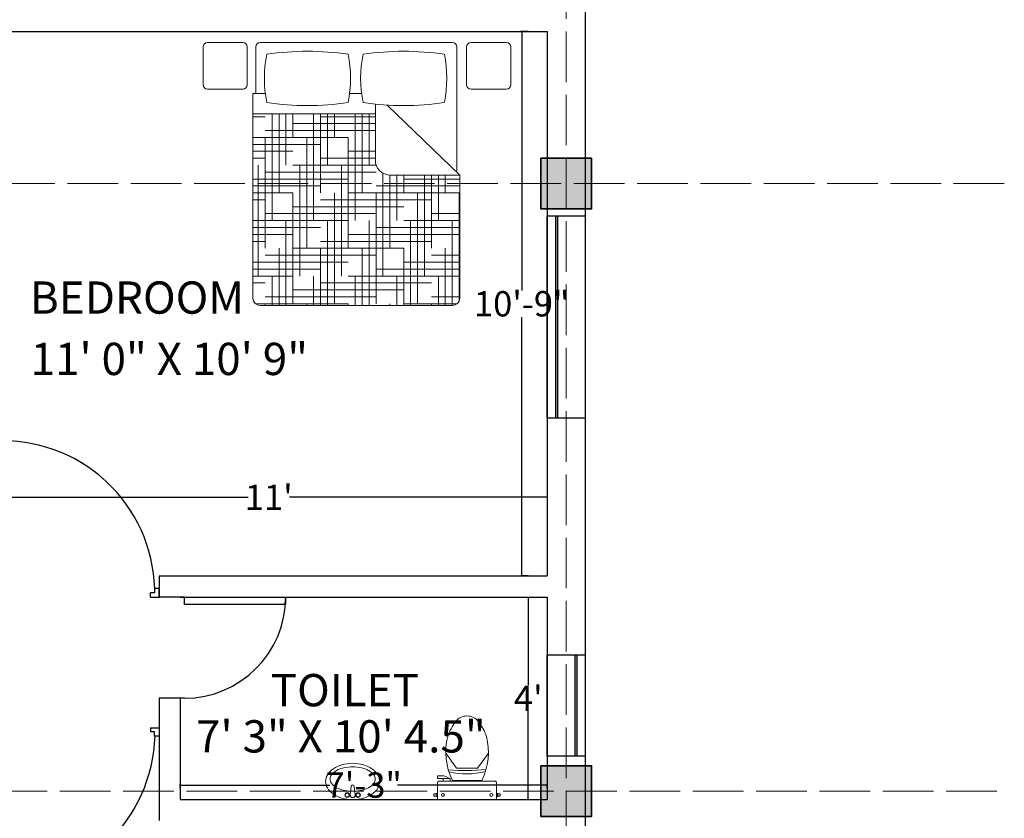
# Model space of a CAD drawing. Units: inches. Extents: x -113 to 5399, y -1393 to 3302.
# Tile 5 of 40: x 1193 to 1427, y 271 to 460. Entities that reach past the tile are written whole.
import ezdxf

# ---------------------------------------------------------------- set-up
doc = ezdxf.new("R2010")
doc.units = ezdxf.units.IN
doc.header["$MEASUREMENT"] = 0
doc.linetypes.add('ACAD_ISO02W100', pattern=[15, 12, -3])
for name, color, linetype, lineweight in [('A-ANNO-DIMS', 254, 'Continuous', 18), ('A-AREA-IDEN', 4, 'Continuous', 18), ('A-COLS', 7, 'Continuous', 35), ('A-FLOR-FIXT', 8, 'Continuous', 18), ('doors', 2, 'Continuous', 25), ('furniture', 131, 'Continuous', 18), ('GRIDS', 7, 'ACAD_ISO02W100', 13), ('walls', 1, 'Continuous', 25), ('windows', 3, 'Continuous', 25)]:
    doc.layers.add(name, color=color, linetype=linetype, lineweight=lineweight)
doc.styles.get("Standard").update_dxf_attribs({"font": 'arial.ttf'})
doc.dimstyles.get("Standard").update_dxf_attribs({"dimtxt": 6, "dimasz": 0.18, "dimexe": 0.18, "dimexo": 0.0625, "dimgap": 0.09, "dimtad": 0, "dimtih": 1, "dimtoh": 1, "dimdec": 1, "dimzin": 0, "dimdsep": 46, "dimlunit": 4, "dimtxsty": 'Standard', "dimblk": 'ARCHTICK', "dimcen": 0.09, "dimadec": 0, "dimazin": 0, "dimtfac": 1, "dimtdec": 1, "dimtofl": 0, "dimtmove": 0, "dimatfit": 3, "dimfxl": 1, "dimtolj": 1, "dimtzin": 0, "dimarcsym": 0})

# ---------------------------------------------------------------- blocks, each defined once
blk = doc.blocks.new('*U2')
for p, q in [((0, 0), (0, -6)), ((24, 0), (24, -6))]:
    blk.add_line(p, q)
blk.add_lwpolyline([(0, 0), (0, 24), (1.75, 24), (1.75, 0)], close=True)
blk.add_arc((0, 0), 24, 0, 90)
blk = doc.blocks.new('*X4')
at = {"color": 0}
for p, q in [((4.3594, 18.5625), (4.3594, 18.6457)), ((4.5, 18), (4.5, 18.6457)), ((4.5469, 18.1875), (4.5469, 18.6457)), ((4.5938, 18.375), (4.5938, 18.6457)), ((4.6406, 18.5625), (4.6406, 18.6457)), ((4.6875, 18.6094), (5.4375, 18.6094)), ((4.7812, 18), (4.7812, 18.6457)), ((4.8281, 18.1875), (4.8281, 18.6457)), ((4.875, 18.375), (4.875, 18.6457)), ((4.9219, 18.5625), (4.9219, 18.6457)), ((5.0625, 18), (5.0625, 18.6457)), ((5.1094, 18.1875), (5.1094, 18.6457)), ((5.1562, 18.375), (5.1562, 18.6457)), ((5.2031, 18.5625), (5.2031, 18.6457)), ((5.3438, 18), (5.3438, 18.6457)), ((5.3906, 18.1875), (5.3906, 18.6457)), ((5.4375, 18.375), (5.4375, 18.6457)), ((5.4844, 18.5625), (5.4844, 18.6457)), ((5.625, 18), (5.625, 18.6287)), ((4.4531, 17.8169), (4.4531, 18.5625)), ((4.5, 18.5625), (5.25, 18.5625)), ((4.7344, 17.8125), (4.7344, 18.5625)), ((5.0156, 17.8125), (5.0156, 18.5625)), ((5.2969, 17.8125), (5.2969, 18.5625)), ((5.5781, 17.8125), (5.5781, 18.5625)), ((5.625, 18.5625), (5.6375, 18.5625)), ((4.3395, 18.5156), (5.0625, 18.5156)), ((4.3395, 18.4688), (4.875, 18.4688)), ((5.25, 18.4688), (5.6375, 18.4688)), ((5.4375, 18.5156), (5.6375, 18.5156)), ((4.3395, 18.4219), (4.6875, 18.4219)), ((5.0625, 18.4219), (5.6375, 18.4219)), ((4.3395, 18.375), (4.5, 18.375)), ((4.4062, 17.8169), (4.4062, 18.375)), ((4.6875, 17.8114), (4.6875, 18.375)), ((4.6875, 18.3281), (5.4375, 18.3281)), ((4.875, 18.375), (5.625, 18.375)), ((4.9688, 17.625), (4.9688, 18.375)), ((5.25, 17.625), (5.25, 18.375)), ((5.5312, 17.625), (5.5312, 18.375)), ((4.5, 18.2812), (5.25, 18.2812)), ((5.625, 18.2812), (5.6375, 18.2812)), ((4.3395, 18.2344), (5.0625, 18.2344)), ((5.4375, 18.2344), (5.6375, 18.2344)), ((4.3395, 18.1875), (4.875, 18.1875)), ((4.3395, 18.1406), (4.6875, 18.1406)), ((4.3594, 17.8169), (4.3594, 18.1875)), ((4.6406, 17.8169), (4.6406, 18.1875)), ((4.9219, 17.4375), (4.9219, 18.1875)), ((5.0625, 18.1406), (5.6375, 18.1406)), ((5.2031, 17.4375), (5.2031, 18.1875)), ((5.25, 18.1875), (5.6375, 18.1875)), ((5.4844, 17.4375), (5.4844, 18.1875)), ((4.3395, 18.0938), (4.5, 18.0938)), ((4.875, 18.0938), (5.625, 18.0938)), ((4.5, 18), (5.25, 18)), ((4.5938, 17.8169), (4.5938, 18)), ((4.6875, 18.0469), (5.4375, 18.0469)), ((4.875, 17.25), (4.875, 18)), ((5.1562, 17.25), (5.1562, 18)), ((5.4375, 17.25), (5.4375, 18)), ((5.625, 18), (5.6375, 18)), ((4.3395, 17.9531), (5.0625, 17.9531)), ((5.4375, 17.9531), (5.6375, 17.9531)), ((4.3395, 17.9062), (4.875, 17.9062)), ((4.3395, 17.8594), (4.6875, 17.8594)), ((5.0625, 17.8594), (5.6375, 17.8594)), ((5.25, 17.9062), (5.6375, 17.9062)), ((4.8281, 17.2457), (4.8281, 17.8125)), ((4.875, 17.8125), (5.625, 17.8125)), ((5.1094, 17.2457), (5.1094, 17.8125)), ((5.3906, 17.2457), (5.3906, 17.8125)), ((4.7421, 17.7656), (5.4375, 17.7656)), ((4.7548, 17.7188), (5.25, 17.7188)), ((4.7548, 17.6719), (5.0625, 17.6719)), ((5.4375, 17.6719), (5.6375, 17.6719)), ((5.625, 17.7188), (5.6375, 17.7188)), ((4.7548, 17.625), (4.875, 17.625)), ((4.7812, 17.2457), (4.7812, 17.625)), ((5.0625, 17.2457), (5.0625, 17.625)), ((5.25, 17.625), (5.6375, 17.625)), ((5.3438, 17.2457), (5.3438, 17.625)), ((5.625, 17.2627), (5.625, 17.625)), ((4.875, 17.5312), (5.625, 17.5312)), ((5.0625, 17.5781), (5.6375, 17.5781)), ((4.7548, 17.4844), (5.4375, 17.4844)), ((4.7548, 17.4375), (5.25, 17.4375)), ((4.7548, 17.3906), (5.0625, 17.3906)), ((5.0156, 17.2457), (5.0156, 17.4375)), ((5.2969, 17.2457), (5.2969, 17.4375)), ((5.4375, 17.3906), (5.6375, 17.3906)), ((5.5781, 17.2457), (5.5781, 17.4375)), ((5.625, 17.4375), (5.6375, 17.4375)), ((4.7548, 17.3438), (4.875, 17.3438)), ((5.25, 17.3438), (5.6375, 17.3438)), ((5.0625, 17.2969), (5.6375, 17.2969)), ((4.875, 17.25), (5.6077, 17.25)), ((4.9688, 17.2457), (4.9688, 17.25)), ((5.25, 17.2457), (5.25, 17.25)), ((5.5312, 17.2457), (5.5312, 17.25))]:
    blk.add_line(p, q, dxfattribs=at)
blk = doc.blocks.new('MAT-P01')
for p, q in [((-0.0213, 0.8164), (-0.0213, 0.5605)), ((0.0087, 0.8464), (0.2471, 0.8464)), ((0.2771, 0.8164), (0.2771, 0.5605)), ((0.3437, 0.8164), (0.3437, -0.0316)), ((0.3737, 0.8464), (1.6737, 0.8464)), ((1.7037, 0.8164), (1.7037, 0.5005)), ((1.7622, 0.8164), (1.7622, 0.5605)), ((1.7922, 0.8464), (2.0306, 0.8464)), ((2.0606, 0.8164), (2.0606, 0.5605)), ((0.0087, 0.5305), (0.2471, 0.5305)), ((0.9879, 0.5005), (1.0693, 0.5005)), ((1.6393, 0.5005), (1.7237, 0.5005)), ((1.7237, 0.5005), (1.7237, -0.8836)), ((1.7922, 0.5305), (2.0306, 0.5305)), ((0.8146, 0.423), (0.3237, -0.0509)), ((0.8949, 0.4293), (0.8949, 0.0491)), ((0.8949, 0.3643), (1.7237, 0.3643)), ((0.8949, 0.3643), (0.8949, 0.0491)), ((0.8949, 0.3643), (1.7237, 0.3643)), ((1.7237, 0.3643), (1.7237, -0.8836)), ((0.3237, -0.0509), (0.7949, -0.0509)), ((0.3237, -0.0509), (0.3237, -0.8836)), ((0.3737, -0.9336), (1.6737, -0.9336))]:
    blk.add_line(p, q)
for centre, radius, start, end in [((0.0087, 0.8164), 0.03, 90, 180), ((0.2471, 0.8164), 0.03, 0, 90), ((0.3737, 0.8164), 0.03, 90, 180), ((1.6737, 0.8164), 0.03, 0, 90), ((1.7922, 0.8164), 0.03, 90, 180), ((2.0306, 0.8164), 0.03, 0, 90), ((1.2251, 0.6034), 0.8138, 168.37298, 191.62702), ((0.7029, -1.1436), 1.9306, 81.81622, 98.18378), ((0.1806, 0.6034), 0.8138, 348.37298, 11.62702), ((1.8766, 0.6034), 0.8138, 168.37298, 191.62702), ((1.3543, -1.1436), 1.9306, 81.81622, 98.18378), ((0.8321, 0.6034), 0.8138, 348.37298, 11.62702), ((0.0087, 0.5605), 0.03, 180, 270), ((0.2471, 0.5605), 0.03, 270, 0), ((1.7922, 0.5605), 0.03, 180, 270), ((2.0306, 0.5605), 0.03, 270, 0), ((0.7029, 2.3504), 1.9306, 261.81622, 278.18378), ((1.3543, 2.3504), 1.9306, 261.81622, 278.18378), ((0.7949, 0.0491), 0.1, 270, 0), ((0.3737, -0.8836), 0.05, 180, 270), ((1.6737, -0.8836), 0.05, 270, 0)]:
    blk.add_arc(centre, radius, start, end)
at = {"rotation": 270}
blk.add_blockref('*X4', (-16.9221, 4.7038), dxfattribs=at)
blk = doc.blocks.new('toilet-3')
at = {"color": 0, "linetype": 'ByBlock'}
for p, q in [((-0.2813, -0.0495), (-0.2813, -0.069)), ((-0.2813, -0.0495), (-0.2613, -0.0495)), ((-0.2813, -0.069), (-0.2613, -0.069)), ((-0.2613, -0.0467), (-0.2613, -0.0717)), ((-0.2613, -0.0467), (-0.2513, -0.0467)), ((-0.2613, -0.0717), (-0.2513, -0.0717)), ((-0.2513, -0.0467), (-0.2513, -0.0717)), ((-0.25, -0.03), (-0.25, -0.1645)), ((0.24, -0.02), (-0.24, -0.02)), ((0.25, -0.03), (0.25, -0.1645)), ((0.2613, -0.0467), (0.2513, -0.0467)), ((0.2513, -0.0467), (0.2513, -0.0717)), ((0.2613, -0.0717), (0.2513, -0.0717)), ((0.2613, -0.0467), (0.2613, -0.0717)), ((0.2813, -0.0495), (0.2613, -0.0495)), ((0.2813, -0.069), (0.2613, -0.069)), ((0.2813, -0.0495), (0.2813, -0.069)), ((-0.1435, -0.1995), (-0.25, -0.1995)), ((-0.25, -0.1995), (-0.25, -0.2221)), ((-0.1981, -0.2221), (-0.25, -0.2221)), ((0.24, -0.1745), (-0.24, -0.1745)), ((-0.2025, -0.1995), (-0.2025, -0.1745)), ((-0.1981, -0.2221), (-0.1601, -0.2072)), ((-0.1601, -0.2072), (-0.1601, -0.1995)), ((-0.1435, -0.1995), (-0.1435, -0.1745)), ((0.125, -0.1821), (-0.125, -0.1821)), ((-0.0886, -0.2874), (-0.1803, -0.4145)), ((0.0886, -0.2874), (-0.0886, -0.2874)), ((0.0886, -0.2874), (0.1803, -0.4145))]:
    blk.add_line(p, q, dxfattribs=at)
for centre in [(-0.2052, -0.0592), (0.2052, -0.0592)]:
    blk.add_circle(centre, 0.0125, dxfattribs=at)
for centre, radius, start, end in [((-0.24, -0.03), 0.01, 90, 180), ((0.24, -0.03), 0.01, 0, 90), ((-0.24, -0.1645), 0.01, 180, 270), ((0.24, -0.1645), 0.01, 270, 0), ((0.3763, -0.4241), 0.5567, 154.23211, 193.67546), ((-0.0054, -0.8958), 0.6585, 75.92762, 103.02045), ((-0.3763, -0.4241), 0.5567, 346.32454, 25.76789), ((-0.013, -1.7868), 1.5207, 83.45525, 95.52712), ((0.2621, -0.4063), 0.4521, 199.29417, 217.25487), ((-0.265, -0.4003), 0.4568, 322.23824, 340.10511), ((-0.0008, -0.6086), 0.1204, 216.37945, 323.62055)]:
    blk.add_arc(centre, radius, start, end, dxfattribs=at)
blk = doc.blocks.new('wash-6')
at = {"color": 0, "linetype": 'ByBlock'}
for p, q in [((-0.036, -0.063), (-0.021, -0.18)), ((0.036, -0.063), (0.021, -0.18))]:
    blk.add_line(p, q, dxfattribs=at)
for centre, radius in [((-0.075, -0.062), 0.0325), ((-0.075, -0.062), 0.0263), ((0.075, -0.062), 0.0325), ((0.075, -0.062), 0.0263)]:
    blk.add_circle(centre, radius, dxfattribs=at)
for centre, radius, start, end in [((0, -0.56), 0.56, 90, 105.4371), ((-0.107, -0.311), 0.285, 123.6901, 148.1465), ((-0.042, -0.407), 0.401, 105.4371, 123.6901), ((-0.045, -0.488), 0.37, 102.6081, 118.369), ((0, -0.69), 0.576, 92.9466, 102.6081), ((0, -0.063), 0.0361, 0, 180), ((0, -0.56), 0.56, 74.5629, 90), ((0, -0.69), 0.576, 77.3919, 87.0534), ((0.045, -0.488), 0.37, 61.631, 77.3919), ((0.042, -0.407), 0.401, 56.3099, 74.5629), ((0.107, -0.311), 0.285, 31.8535, 56.3099), ((-0.204, -0.25), 0.17, 148.1465, 180), ((-0.204, -0.25), 0.17, 180, 211.8535), ((-0.217, -0.282), 0.0954, 142.5096, 180), ((-0.114, -0.361), 0.225, 118.369, 142.5096), ((0, -0.18), 0.0215, 180, 0), ((0.114, -0.361), 0.225, 37.4904, 61.631), ((0.217, -0.282), 0.0954, 0, 37.4904), ((0.204, -0.25), 0.17, 0, 31.8535), ((0.204, -0.25), 0.17, 328.1465, 0), ((-0.107, -0.189), 0.285, 211.8535, 236.3099), ((-0.217, -0.282), 0.0954, 180, 217.4904), ((-0.114, -0.203), 0.225, 217.4904, 241.631), ((-0.045, -0.076), 0.37, 241.631, 257.3919), ((0.045, -0.076), 0.37, 282.6081, 298.369), ((0.114, -0.203), 0.225, 298.369, 322.5096), ((0.107, -0.189), 0.285, 303.6901, 328.1465), ((0.217, -0.282), 0.0954, 322.5096, 0), ((-0.042, -0.092), 0.401, 236.3099, 254.5629), ((0, 0.06), 0.56, 254.5629, 270), ((0, 0.125), 0.576, 257.3919, 270), ((0, 0.125), 0.576, 270, 282.6081), ((0, 0.06), 0.56, 270, 285.4371), ((0.042, -0.092), 0.401, 285.4371, 303.6901)]:
    blk.add_arc(centre, radius, start, end, dxfattribs=at)
blk = doc.blocks.new('_ArchTick')
at = {"color": 0, "linetype": 'ByBlock', "const_width": 0.15}
blk.add_lwpolyline([(-0.5, -0.5), (0.5, 0.5)], dxfattribs=at)
blk = doc.blocks.new('*D41')
at = {"layer": 'A-ANNO-DIMS', "color": 0, "lineweight": -2, "transparency": 16777216}
for p, q in [((1313.73, 323.03), (1313.73, 302.12)), ((1313.75, 323.03), (1313.91, 323.03)), ((1313.73, 275.03), (1313.73, 295.94)), ((1313.75, 275.03), (1313.91, 275.03))]:
    blk.add_line(p, q, dxfattribs=at)
at = {"layer": 'Defpoints', "color": 0, "transparency": 16777216}
for p in [(1313.68, 323.03), (1313.68, 275.03), (1313.73, 275.03)]:
    blk.add_point(p, dxfattribs=at)
at = {"layer": 'A-ANNO-DIMS', "color": 0, "lineweight": -2, "transparency": 16777216, "xscale": 0.18, "yscale": 0.18, "zscale": 0.18}
for p, rotation in [((1313.73, 323.03), 90), ((1313.73, 275.03), 270)]:
    blk.add_blockref('_ArchTick', p, dxfattribs=dict(at, rotation=rotation))
at = {"layer": 'A-ANNO-DIMS', "color": 0, "transparency": 16777216, "insert": (1313.73, 299.03), "char_height": 6, "attachment_point": 5}
blk.add_mtext("\\A1;4'", dxfattribs=at)
blk = doc.blocks.new('*D42')
at = {"layer": 'A-ANNO-DIMS', "color": 0, "lineweight": -2, "transparency": 16777216}
for p, q in [((1231.23, 277.83), (1231.23, 278.64)), ((1231.23, 278.46), (1266.69, 278.46)), ((1318.23, 278.46), (1282.77, 278.46)), ((1318.23, 277.83), (1318.23, 278.64))]:
    blk.add_line(p, q, dxfattribs=at)
at = {"layer": 'Defpoints', "color": 0, "transparency": 16777216}
for p in [(1231.23, 278.46), (1231.23, 277.77), (1318.23, 277.77)]:
    blk.add_point(p, dxfattribs=at)
at = {"layer": 'A-ANNO-DIMS', "color": 0, "lineweight": -2, "transparency": 16777216, "xscale": 0.18, "yscale": 0.18, "zscale": 0.18, "rotation": 180}
blk.add_blockref('_ArchTick', (1231.23, 278.46), dxfattribs=at)
at = {"layer": 'A-ANNO-DIMS', "color": 0, "lineweight": -2, "transparency": 16777216, "xscale": 0.18, "yscale": 0.18, "zscale": 0.18}
blk.add_blockref('_ArchTick', (1318.23, 278.46), dxfattribs=at)
at = {"layer": 'A-ANNO-DIMS', "color": 0, "transparency": 16777216, "insert": (1274.73, 278.46), "char_height": 6, "attachment_point": 5}
blk.add_mtext('\\A1;7\'-3"', dxfattribs=at)
blk = doc.blocks.new('*D43')
at = {"layer": 'A-ANNO-DIMS', "color": 0, "lineweight": -2, "transparency": 16777216}
for p, q in [((1313.68, 457.03), (1311.99, 457.03)), ((1312.17, 457.03), (1312.17, 395.69)), ((1312.17, 328.03), (1312.17, 389.38)), ((1313.68, 328.03), (1311.99, 328.03))]:
    blk.add_line(p, q, dxfattribs=at)
at = {"layer": 'Defpoints', "color": 0, "transparency": 16777216}
for p in [(1313.74, 457.03), (1312.17, 328.03), (1313.74, 328.03)]:
    blk.add_point(p, dxfattribs=at)
at = {"layer": 'A-ANNO-DIMS', "color": 0, "lineweight": -2, "transparency": 16777216, "xscale": 0.18, "yscale": 0.18, "zscale": 0.18}
for p, rotation in [((1312.17, 457.03), 90), ((1312.17, 328.03), 270)]:
    blk.add_blockref('_ArchTick', p, dxfattribs=dict(at, rotation=rotation))
at = {"layer": 'A-ANNO-DIMS', "color": 0, "transparency": 16777216, "insert": (1312.17, 392.53), "char_height": 6, "attachment_point": 5}
blk.add_mtext('\\A1;10\'-9"', dxfattribs=at)
blk = doc.blocks.new('*D44')
at = {"layer": 'A-ANNO-DIMS', "color": 0, "lineweight": -2, "transparency": 16777216}
for p, q in [((1186.23, 346.73), (1186.23, 346.84)), ((1186.23, 346.66), (1247.33, 346.66)), ((1318.23, 346.66), (1257.13, 346.66)), ((1318.23, 346.73), (1318.23, 346.84))]:
    blk.add_line(p, q, dxfattribs=at)
at = {"layer": 'Defpoints', "color": 0, "transparency": 16777216}
for p in [(1186.23, 346.66), (1186.23, 346.66), (1318.23, 346.66)]:
    blk.add_point(p, dxfattribs=at)
at = {"layer": 'A-ANNO-DIMS', "color": 0, "lineweight": -2, "transparency": 16777216, "xscale": 0.18, "yscale": 0.18, "zscale": 0.18, "rotation": 180}
blk.add_blockref('_ArchTick', (1186.23, 346.66), dxfattribs=at)
at = {"layer": 'A-ANNO-DIMS', "color": 0, "lineweight": -2, "transparency": 16777216, "xscale": 0.18, "yscale": 0.18, "zscale": 0.18}
blk.add_blockref('_ArchTick', (1318.23, 346.66), dxfattribs=at)
at = {"layer": 'A-ANNO-DIMS', "color": 0, "transparency": 16777216, "insert": (1252.23, 346.66), "char_height": 6, "attachment_point": 5}
blk.add_mtext("\\A1;11'", dxfattribs=at)
blk = doc.blocks.new('WIN-PLAN-48IN')
h = blk.add_hatch(color=256)
h.dxf.hatch_style = 1
h.paths.add_polyline_path([(48, 2.5), (0, 2.5), (0, 2), (48, 2)])
for p, q in [((0, 9), (48, 9)), ((0, 0), (0, 9)), ((48, 9), (48, 0)), ((48, 2.5), (0, 2.5)), ((48, 2), (0, 2)), ((48, 0), (0, 0))]:
    blk.add_line(p, q)
blk = doc.blocks.new('WIN-PLAN-24IN')
h = blk.add_hatch(color=256)
h.dxf.hatch_style = 1
h.paths.add_polyline_path([(6.5, 24), (6.5, 0), (7, 0), (7, 24)])
for p, q in [((0, 0), (0, 24)), ((0, 24), (9, 24)), ((6.5, 24), (6.5, 0)), ((7, 24), (7, 0)), ((9, 24), (9, 0)), ((9, 0), (0, 0))]:
    blk.add_line(p, q)
blk = doc.blocks.new('COLUMN-12IN-SQUARE')
h = blk.add_hatch(color=256)
h.dxf.hatch_style = 1
h.paths.add_polyline_path([(6, 6), (-6, 6), (-6, -6), (6, -6)])
blk.add_lwpolyline([(-6, 6), (6, 6), (6, -6), (-6, -6)], close=True)
blk = doc.blocks.new('DOOR-SINGLE-36IN-PLAN')
for p, q in [((0.5, 2), (0.5, 36.98)), ((0.5, 36.98), (1.5, 36.98)), ((1.5, 36.98), (1.5, 2)), ((0, 2), (0, 0)), ((0, 2), (1.04, 2)), ((1.5, 2), (0.5, 2)), ((1.04, 2), (1.04, 0.98)), ((1.04, 0.98), (2, 0.98)), ((2, 0), (2, 0.98)), ((38.96, 0.98), (38, 0.98)), ((38, 0), (38, 0.98)), ((40, 2), (38.96, 2)), ((38.96, 2), (38.96, 0.98)), ((40, 0), (40, 2)), ((0, 0), (2, 0)), ((0, 0), (2, 0)), ((38, 0), (40, 0))]:
    blk.add_line(p, q)
blk.add_arc((2.94, 0.99), 36.04, 1.6003, 93.0893)

msp = doc.modelspace()

# ---------------------------------------------------------------- linework, layer by layer
at = {"layer": 'GRIDS'}
for p, q in [((1322.73, 922.09), (1322.73, 54.5)), ((1426.54, 421.03), (768.3, 421.03)), ((767.75, 277.03), (1426.54, 277.03))]:
    msp.add_line(p, q, dxfattribs=at)
at = {"layer": 'walls'}
for p, q in [((1327.23, 786.53), (1327.23, 136.53)), ((1169.23, 457.03), (1318.23, 457.03)), ((1318.23, 457.03), (1318.23, 332.53)), ((1318.23, 332.53), (1318.23, 328.03)), ((1226.23, 328.03), (1226.23, 323.03)), ((1226.23, 328.03), (1318.23, 328.03)), ((1231.23, 323.03), (1226.23, 323.03)), ((1231.23, 323.03), (1318.23, 323.03)), ((1318.23, 323.03), (1318.23, 275.03)), ((1226.23, 299.03), (1226.23, 270.03)), ((1231.23, 299.03), (1226.23, 299.03)), ((1231.23, 299.03), (1231.23, 275.03)), ((1231.23, 275.03), (1318.23, 275.03))]:
    msp.add_line(p, q, dxfattribs=at)

# ---------------------------------------------------------------- block references
at = {"layer": 'A-COLS'}
for p in [(1322.73, 421.03), (1322.73, 277.03)]:
    msp.add_blockref('COLUMN-12IN-SQUARE', p, dxfattribs=at)
at = {"layer": 'A-FLOR-FIXT', "rotation": 180}
for name, p, xscale, yscale, zscale in [('toilet-3', (1299.23, 274.47), -27.95492935005888, 27.95492935005888, 27.95492935005888), ('wash-6', (1272.11, 275.03), -17.16666334294967, 17.16666334294967, 17.16666334294967)]:
    msp.add_blockref(name, p, dxfattribs=dict(at, xscale=xscale, yscale=yscale, zscale=zscale))
at = {"layer": 'doors'}
msp.add_blockref('DOOR-SINGLE-36IN-PLAN', (1186.23, 323.03), dxfattribs=at)
at = {"layer": 'doors', "rotation": 270}
msp.add_blockref('*U2', (1232.23, 323.03), dxfattribs=at)
at = {"layer": 'doors', "extrusion": (0, 0, -1), "zscale": -1, "rotation": 180}
msp.add_blockref('DOOR-SINGLE-36IN-PLAN', (-1186.23, 292.03), dxfattribs=at)
at = {"layer": 'furniture', "xscale": -35.02364872074636, "yscale": 35.02364872074636, "zscale": 35.02364872074636}
msp.add_blockref('MAT-P01', (1308.83, 424.81), dxfattribs=at)
at = {"layer": 'windows', "rotation": 269.9999999999989}
msp.add_blockref('WIN-PLAN-48IN', (1318.23, 413.39), dxfattribs=at)
at = {"layer": 'windows'}
msp.add_blockref('WIN-PLAN-24IN', (1318.23, 285.31), dxfattribs=at)

# ---------------------------------------------------------------- texts
at = {"layer": 'A-AREA-IDEN'}
for s, height, p in [('BEDROOM', 7.647, (1195.62, 390.18)), ('11\' 0" X 10\' 9"', 7.6473, (1195.79, 375.64)), ('TOILET', 7.647, (1252.7, 297.13)), ('7\' 3" X 10\' 4.5"', 7.6473, (1234.99, 286.18))]:
    msp.add_text(s, height=height, dxfattribs=at).set_placement(p)

# ---------------------------------------------------------------- dimensions: what is measured, and where the dimension line sits
at = {"layer": 'A-ANNO-DIMS'}
for base, p1, p2, picture, middle in [((1312.17, 328.03), (1313.74, 457.03), (1313.74, 328.03), '*D43', (1312.17, 392.53)), ((1313.73, 275.03), (1313.68, 323.03), (1313.68, 275.03), '*D41', (1313.73, 299.03))]:
    dim = msp.add_linear_dim(base=base, p1=p1, p2=p2, angle=90, dimstyle='Standard', override={"dimclrd": 0, "dimclre": 0, "dimclrt": 0}, dxfattribs=at)
    dim.commit()
    dim.dimension.update_dxf_attribs({"geometry": picture, "text_midpoint": middle})
for base, p1, p2, picture, middle in [((1186.23, 346.66), (1318.23, 346.66), (1186.23, 346.66), '*D44', (1252.23, 346.66)), ((1231.23, 278.46), (1318.23, 277.77), (1231.23, 277.77), '*D42', (1274.73, 278.46))]:
    dim = msp.add_linear_dim(base=base, p1=p1, p2=p2, dimstyle='Standard', override={"dimclrd": 0, "dimclre": 0, "dimclrt": 0}, dxfattribs=at)
    dim.commit()
    dim.dimension.update_dxf_attribs({"geometry": picture, "text_midpoint": middle})

doc.saveas('drawing.dxf')
